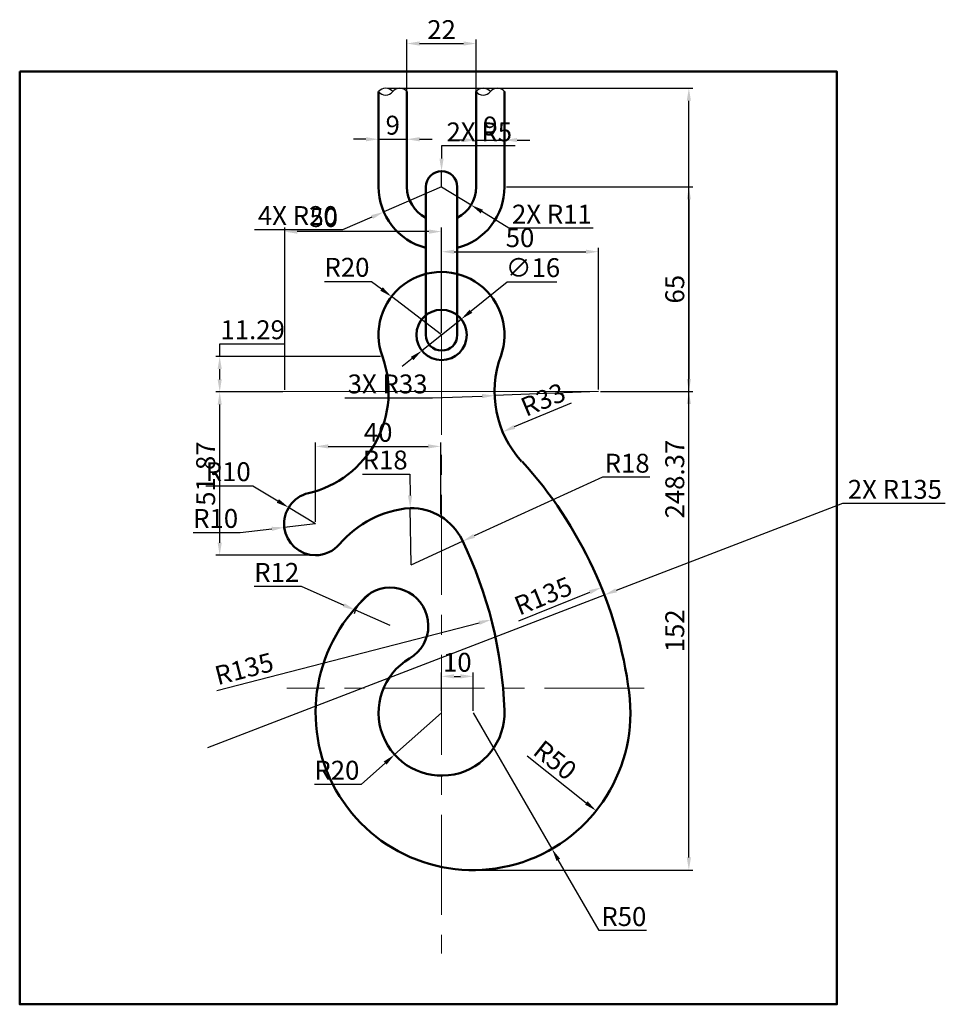
# Model space of a CAD drawing. Units: millimetres. Extents: x 103 to 397, y -55 to 258.
import ezdxf

# ---------------------------------------------------------------- set-up
doc = ezdxf.new("R2010")
doc.units = ezdxf.units.MM
doc.linetypes.add('CENTER', pattern=[50.8, 31.75, -6.35, 6.35, -6.35])
for name, color, linetype, lineweight in [('M-BRKL', 7, 'Continuous', 25), ('M-CNTR', 4, 'CENTER', 18), ('M-CONS', 8, 'Continuous', 18), ('M-DIMS', 2, 'Continuous', 25), ('M-OUTL', 7, 'Continuous', 50), ('M-TTLB', 7, 'Continuous', 50)]:
    doc.layers.add(name, color=color, linetype=linetype, lineweight=lineweight)
doc.styles.get("Standard").update_dxf_attribs({"font": 'arial.ttf'})
doc.dimstyles.new('ISO-25', dxfattribs={"dimtxt": 6, "dimasz": 4, "dimexe": 1.25, "dimexo": 0.625, "dimtad": 1, "dimtoh": 1, "dimdec": 0, "dimtxsty": 'Standard', "dimcen": 2.5, "dimadec": 0, "dimazin": 0, "dimtfac": 1, "dimtdec": 0, "dimtmove": 0, "dimatfit": 3, "dimfxl": 1, "dimarcsym": 0})

# ---------------------------------------------------------------- blocks, each defined once
blk = doc.blocks.new('*D1')
at = {"layer": 'Defpoints', "color": 0, "transparency": 16777216}
for p in [(286.8, 139.63), (256.38, 126.83)]:
    blk.add_point(p, dxfattribs=at)
at = {"layer": 'M-DIMS', "color": 0, "lineweight": -2, "transparency": 16777216}
blk.add_line((278.12, 135.98), (260.06, 128.38), dxfattribs=at)
at = {"layer": 'M-DIMS', "color": 0, "transparency": 16777216}
blk.add_solid([(259.81, 129), (260.32, 127.77), (256.38, 126.83)], dxfattribs=at)
at = {"layer": 'M-DIMS', "color": 0, "transparency": 16777216, "insert": (269.5, 136.36), "char_height": 6, "attachment_point": 5, "rotation": 22.8118}
blk.add_mtext('R33', dxfattribs=at)
blk = doc.blocks.new('*D2')
at = {"layer": 'Defpoints', "color": 0, "transparency": 16777216}
for p in [(287.73, 77.42), (162.67, 26.58)]:
    blk.add_point(p, dxfattribs=at)
at = {"layer": 'M-DIMS', "color": 0, "lineweight": -2, "transparency": 16777216}
blk.add_line((261.52, 66.77), (284.02, 75.92), dxfattribs=at)
at = {"layer": 'M-DIMS', "color": 0, "transparency": 16777216}
blk.add_solid([(283.77, 76.53), (284.27, 75.3), (287.73, 77.42)], dxfattribs=at)
at = {"layer": 'M-DIMS', "color": 0, "transparency": 16777216, "insert": (269.53, 74.01), "char_height": 6, "attachment_point": 5, "rotation": 22.1218}
blk.add_mtext('R135', dxfattribs=at)
blk = doc.blocks.new('*D3')
at = {"layer": 'Defpoints', "color": 0, "transparency": 16777216}
for p in [(246.95, 37.63), (286.06, 6.48)]:
    blk.add_point(p, dxfattribs=at)
at = {"layer": 'M-DIMS', "color": 0, "lineweight": -2, "transparency": 16777216}
blk.add_line((264.16, 23.92), (282.93, 8.97), dxfattribs=at)
at = {"layer": 'M-DIMS', "color": 0, "transparency": 16777216}
blk.add_solid([(283.35, 9.5), (282.52, 8.45), (286.06, 6.48)], dxfattribs=at)
at = {"layer": 'M-DIMS', "color": 0, "transparency": 16777216, "insert": (272.54, 21.96), "char_height": 6, "attachment_point": 5, "rotation": 321.473}
blk.add_mtext('R50', dxfattribs=at)
blk = doc.blocks.new('*D4')
at = {"layer": 'Defpoints', "color": 0, "transparency": 16777216}
for p in [(236.95, 37.63), (222.03, 24.3)]:
    blk.add_point(p, dxfattribs=at)
at = {"layer": 'M-DIMS', "color": 0, "lineweight": -2, "transparency": 16777216}
for p, q in [((236.95, 37.63), (222.03, 24.3)), ((211.49, 14.89), (219.05, 21.64)), ((196.55, 14.89), (211.49, 14.89))]:
    blk.add_line(p, q, dxfattribs=at)
at = {"layer": 'M-DIMS', "color": 0, "transparency": 16777216}
blk.add_solid([(218.6, 22.14), (219.49, 21.14), (222.03, 24.3)], dxfattribs=at)
at = {"layer": 'M-DIMS', "color": 0, "transparency": 16777216, "insert": (203.71, 18.58), "char_height": 6, "attachment_point": 5}
blk.add_mtext('R20', dxfattribs=at)
blk = doc.blocks.new('*D5')
at = {"layer": 'Defpoints', "color": 0, "transparency": 16777216}
for p in [(188.39, 102.8), (196.95, 97.63)]:
    blk.add_point(p, dxfattribs=at)
at = {"layer": 'M-DIMS', "color": 0, "lineweight": -2, "transparency": 16777216}
for p, q in [((162.04, 109.7), (176.98, 109.7)), ((176.98, 109.7), (184.97, 104.87)), ((196.95, 97.63), (188.39, 102.8))]:
    blk.add_line(p, q, dxfattribs=at)
at = {"layer": 'M-DIMS', "color": 0, "transparency": 16777216}
blk.add_solid([(185.31, 105.44), (184.62, 104.3), (188.39, 102.8)], dxfattribs=at)
at = {"layer": 'M-DIMS', "color": 0, "transparency": 16777216, "insert": (169.2, 113.39), "char_height": 6, "attachment_point": 5}
blk.add_mtext('R10', dxfattribs=at)
blk = doc.blocks.new('*D6')
at = {"layer": 'Defpoints', "color": 0, "transparency": 16777216}
for p in [(243.64, 92.1), (227.27, 84.63)]:
    blk.add_point(p, dxfattribs=at)
at = {"layer": 'M-DIMS', "color": 0, "lineweight": -2, "transparency": 16777216}
for p, q in [((288.1, 112.4), (247.28, 93.76)), ((303.07, 112.4), (288.1, 112.4)), ((227.27, 84.63), (243.64, 92.1))]:
    blk.add_line(p, q, dxfattribs=at)
blk.add_arc((227.27, 84.63), 18, 20.5586, 25.8976, dxfattribs=at)
at = {"layer": 'M-DIMS', "color": 0, "transparency": 16777216}
blk.add_solid([(247.01, 94.37), (247.56, 93.16), (243.64, 92.1)], dxfattribs=at)
at = {"layer": 'M-DIMS', "color": 0, "transparency": 16777216, "insert": (295.9, 116.09), "char_height": 6, "attachment_point": 5}
blk.add_mtext('R18', dxfattribs=at)
blk = doc.blocks.new('*D7')
at = {"layer": 'Defpoints', "color": 0, "transparency": 16777216}
for p in [(246.95, 49.17), (236.95, 37.63), (246.95, 37.63)]:
    blk.add_point(p, dxfattribs=at)
at = {"layer": 'M-DIMS', "color": 0, "lineweight": -2, "transparency": 16777216}
for p, q in [((236.95, 38.25), (236.95, 50.42)), ((246.95, 38.25), (246.95, 50.42)), ((240.95, 49.17), (242.95, 49.17))]:
    blk.add_line(p, q, dxfattribs=at)
at = {"layer": 'M-DIMS', "color": 0, "transparency": 16777216}
for points in [[(240.95, 49.84), (240.95, 48.5), (236.95, 49.17)], [(242.95, 49.84), (242.95, 48.5), (246.95, 49.17)]]:
    blk.add_solid(points, dxfattribs=at)
at = {"layer": 'M-DIMS', "color": 0, "transparency": 16777216, "insert": (241.95, 52.86), "char_height": 6, "attachment_point": 5}
blk.add_mtext('10', dxfattribs=at)
blk = doc.blocks.new('*D8')
at = {"layer": 'Defpoints', "color": 0, "transparency": 16777216}
for p in [(216.95, 219.76), (225.95, 219.76), (225.95, 219.76)]:
    blk.add_point(p, dxfattribs=at)
at = {"layer": 'M-DIMS', "color": 0, "lineweight": -2, "transparency": 16777216}
for p, q in [((212.95, 219.76), (208.95, 219.76)), ((216.95, 220.39), (216.95, 221.01)), ((216.95, 219.76), (225.95, 219.76)), ((225.95, 220.39), (225.95, 221.01)), ((229.95, 219.76), (233.95, 219.76))]:
    blk.add_line(p, q, dxfattribs=at)
at = {"layer": 'M-DIMS', "color": 0, "transparency": 16777216}
for points in [[(212.95, 220.43), (212.95, 219.09), (216.95, 219.76)], [(229.95, 220.43), (229.95, 219.09), (225.95, 219.76)]]:
    blk.add_solid(points, dxfattribs=at)
at = {"layer": 'M-DIMS', "color": 0, "transparency": 16777216, "insert": (221.45, 223.45), "char_height": 6, "attachment_point": 5}
blk.add_mtext('9', dxfattribs=at)
blk = doc.blocks.new('*D9')
at = {"layer": 'Defpoints', "color": 0, "transparency": 16777216}
for p in [(247.95, 219.76), (256.95, 219.76), (256.95, 219.5)]:
    blk.add_point(p, dxfattribs=at)
at = {"layer": 'M-DIMS', "color": 0, "lineweight": -2, "transparency": 16777216}
for p, q in [((243.95, 219.5), (239.95, 219.5)), ((247.95, 219.5), (256.95, 219.5)), ((247.95, 219.14), (247.95, 218.25)), ((256.95, 219.14), (256.95, 218.25)), ((260.95, 219.5), (264.95, 219.5))]:
    blk.add_line(p, q, dxfattribs=at)
at = {"layer": 'M-DIMS', "color": 0, "transparency": 16777216}
for points in [[(243.95, 220.17), (243.95, 218.84), (247.95, 219.5)], [(260.95, 220.17), (260.95, 218.84), (256.95, 219.5)]]:
    blk.add_solid(points, dxfattribs=at)
at = {"layer": 'M-DIMS', "color": 0, "transparency": 16777216, "insert": (252.45, 223.19), "char_height": 6, "attachment_point": 5}
blk.add_mtext('9', dxfattribs=at)
blk = doc.blocks.new('*D10')
at = {"layer": 'Defpoints', "color": 0, "transparency": 16777216}
for p in [(243.19, 162.63), (230.7, 152.62)]:
    blk.add_point(p, dxfattribs=at)
at = {"layer": 'M-DIMS', "color": 0, "lineweight": -2, "transparency": 16777216}
for p, q in [((257.81, 174.36), (246.31, 165.13)), ((273.55, 174.36), (257.81, 174.36)), ((230.7, 152.62), (243.19, 162.63)), ((227.58, 150.12), (224.46, 147.62))]:
    blk.add_line(p, q, dxfattribs=at)
at = {"layer": 'M-DIMS', "color": 0, "transparency": 16777216}
for points in [[(245.89, 165.65), (246.72, 164.61), (243.19, 162.63)], [(227.17, 150.64), (228, 149.6), (230.7, 152.62)]]:
    blk.add_solid(points, dxfattribs=at)
at = {"layer": 'M-DIMS', "color": 0, "transparency": 16777216, "insert": (265.99, 178.21), "char_height": 6, "attachment_point": 5}
blk.add_mtext('∅16', dxfattribs=at)
blk = doc.blocks.new('*D11')
at = {"layer": 'Defpoints', "color": 0, "transparency": 16777216}
for p in [(221.05, 169.77), (236.95, 157.63)]:
    blk.add_point(p, dxfattribs=at)
at = {"layer": 'M-DIMS', "color": 0, "lineweight": -2, "transparency": 16777216}
for p, q in [((199.75, 174.62), (214.7, 174.62)), ((214.7, 174.62), (217.87, 172.2)), ((236.95, 157.63), (221.05, 169.77))]:
    blk.add_line(p, q, dxfattribs=at)
at = {"layer": 'M-DIMS', "color": 0, "transparency": 16777216}
blk.add_solid([(218.28, 172.73), (217.47, 171.67), (221.05, 169.77)], dxfattribs=at)
at = {"layer": 'M-DIMS', "color": 0, "transparency": 16777216, "insert": (206.91, 178.31), "char_height": 6, "attachment_point": 5}
blk.add_mtext('R20', dxfattribs=at)
blk = doc.blocks.new('*D12')
at = {"layer": 'Defpoints', "color": 0, "transparency": 16777216}
for p in [(236.68, 122.21), (196.95, 97.63), (236.68, 99.97)]:
    blk.add_point(p, dxfattribs=at)
at = {"layer": 'M-DIMS', "color": 0, "lineweight": -2, "transparency": 16777216}
for p, q in [((196.95, 98.25), (196.95, 123.46)), ((200.95, 122.21), (232.68, 122.21)), ((236.68, 100.59), (236.68, 123.46))]:
    blk.add_line(p, q, dxfattribs=at)
at = {"layer": 'M-DIMS', "color": 0, "transparency": 16777216}
for points in [[(200.95, 122.88), (200.95, 121.54), (196.95, 122.21)], [(232.68, 122.88), (232.68, 121.54), (236.68, 122.21)]]:
    blk.add_solid(points, dxfattribs=at)
at = {"layer": 'M-DIMS', "color": 0, "transparency": 16777216, "insert": (216.81, 125.9), "char_height": 6, "attachment_point": 5}
blk.add_mtext('40', dxfattribs=at)
blk = doc.blocks.new('*D13')
at = {"layer": 'Defpoints', "color": 0, "transparency": 16777216}
for p in [(286.8, 184.04), (236.95, 157.63), (286.8, 139.63)]:
    blk.add_point(p, dxfattribs=at)
at = {"layer": 'M-DIMS', "color": 0, "lineweight": -2, "transparency": 16777216}
for p, q in [((236.95, 158.25), (236.95, 185.29)), ((286.8, 140.25), (286.8, 185.29)), ((240.95, 184.04), (282.8, 184.04))]:
    blk.add_line(p, q, dxfattribs=at)
at = {"layer": 'M-DIMS', "color": 0, "transparency": 16777216}
for points in [[(240.95, 184.7), (240.95, 183.37), (236.95, 184.04)], [(282.8, 184.7), (282.8, 183.37), (286.8, 184.04)]]:
    blk.add_solid(points, dxfattribs=at)
at = {"layer": 'M-DIMS', "color": 0, "transparency": 16777216, "insert": (261.87, 187.72), "char_height": 6, "attachment_point": 5}
blk.add_mtext('50', dxfattribs=at)
blk = doc.blocks.new('*D14')
at = {"layer": 'Defpoints', "color": 0, "transparency": 16777216}
for p in [(187.14, 190.43), (236.95, 157.63), (187.14, 139.49)]:
    blk.add_point(p, dxfattribs=at)
at = {"layer": 'M-DIMS', "color": 0, "lineweight": -2, "transparency": 16777216}
for p, q in [((187.14, 140.12), (187.14, 191.68)), ((236.95, 158.25), (236.95, 191.68)), ((232.95, 190.43), (191.14, 190.43))]:
    blk.add_line(p, q, dxfattribs=at)
at = {"layer": 'M-DIMS', "color": 0, "transparency": 16777216}
for points in [[(191.14, 191.09), (191.14, 189.76), (187.14, 190.43)], [(232.95, 191.09), (232.95, 189.76), (236.95, 190.43)]]:
    blk.add_solid(points, dxfattribs=at)
at = {"layer": 'M-DIMS', "color": 0, "transparency": 16777216, "insert": (199.54, 194.12), "char_height": 6, "attachment_point": 5}
blk.add_mtext('50', dxfattribs=at)
blk = doc.blocks.new('*D15')
at = {"layer": 'Defpoints', "color": 0, "transparency": 16777216}
for p in [(209.6, 70.15), (220.65, 65.27)]:
    blk.add_point(p, dxfattribs=at)
at = {"layer": 'M-DIMS', "color": 0, "lineweight": -2, "transparency": 16777216}
for p, q in [((177.45, 77.77), (192.35, 77.77)), ((192.35, 77.77), (205.94, 71.77)), ((220.65, 65.27), (209.6, 70.15))]:
    blk.add_line(p, q, dxfattribs=at)
blk.add_arc((220.65, 65.27), 12.09, 123.4798, 162.0881, dxfattribs=at)
at = {"layer": 'M-DIMS', "color": 0, "transparency": 16777216}
blk.add_solid([(206.21, 72.38), (205.67, 71.16), (209.6, 70.15)], dxfattribs=at)
at = {"layer": 'M-DIMS', "color": 0, "transparency": 16777216, "insert": (184.59, 81.41), "char_height": 6, "attachment_point": 5}
blk.add_mtext('R12', dxfattribs=at)
blk = doc.blocks.new('*D16')
at = {"layer": 'Defpoints', "color": 0, "transparency": 16777216}
for p in [(252.76, 67.17), (122.02, 33.53)]:
    blk.add_point(p, dxfattribs=at)
at = {"layer": 'M-DIMS', "color": 0, "lineweight": -2, "transparency": 16777216}
blk.add_line((165.54, 44.72), (248.89, 66.17), dxfattribs=at)
at = {"layer": 'M-DIMS', "color": 0, "transparency": 16777216}
blk.add_solid([(248.72, 66.82), (249.05, 65.53), (252.76, 67.17)], dxfattribs=at)
at = {"layer": 'M-DIMS', "color": 0, "transparency": 16777216, "insert": (174.44, 50.83), "char_height": 6, "attachment_point": 5, "rotation": 14.4308}
blk.add_mtext('R135', dxfattribs=at)
blk = doc.blocks.new('FORK-ARM-BREAK-9')
for centre, start, end in [((2.25, -0.61), 37.4068, 142.5932), ((2.25, 2.83), 217.4068, 322.5932), ((6.75, -0.61), 37.4068, 142.5932)]:
    blk.add_arc(centre, 2.83, start, end)
blk = doc.blocks.new('*D18')
at = {"layer": 'Defpoints', "color": 0, "transparency": 16777216}
for p in [(219.2, 236.01), (315.49, 236.01), (245.57, -12.36)]:
    blk.add_point(p, dxfattribs=at)
at = {"layer": 'M-DIMS', "color": 0, "lineweight": -2, "transparency": 16777216}
for p, q in [((219.82, 236.01), (316.74, 236.01)), ((315.49, -8.36), (315.49, 232.01)), ((246.2, -12.36), (316.74, -12.36))]:
    blk.add_line(p, q, dxfattribs=at)
at = {"layer": 'M-DIMS', "color": 0, "transparency": 16777216}
for points in [[(314.83, 232.01), (316.16, 232.01), (315.49, 236.01)], [(314.83, -8.36), (316.16, -8.36), (315.49, -12.36)]]:
    blk.add_solid(points, dxfattribs=at)
at = {"layer": 'M-DIMS', "color": 0, "transparency": 16777216, "insert": (311.8, 111.82), "char_height": 6, "attachment_point": 5, "rotation": 90}
blk.add_mtext('248.37', dxfattribs=at)
blk = doc.blocks.new('*D19')
at = {"layer": 'Defpoints', "color": 0, "transparency": 16777216}
for p in [(166.49, 139.49), (187.14, 139.49), (196.95, 87.63)]:
    blk.add_point(p, dxfattribs=at)
at = {"layer": 'M-DIMS', "color": 0, "lineweight": -2, "transparency": 16777216}
for p, q in [((186.52, 139.49), (165.24, 139.49)), ((166.49, 91.63), (166.49, 135.49)), ((196.32, 87.63), (165.24, 87.63))]:
    blk.add_line(p, q, dxfattribs=at)
at = {"layer": 'M-DIMS', "color": 0, "transparency": 16777216}
for points in [[(165.82, 135.49), (167.15, 135.49), (166.49, 139.49)], [(165.82, 91.63), (167.15, 91.63), (166.49, 87.63)]]:
    blk.add_solid(points, dxfattribs=at)
at = {"layer": 'M-DIMS', "color": 0, "transparency": 16777216, "insert": (162.8, 113.56), "char_height": 6, "attachment_point": 5, "rotation": 90}
blk.add_mtext('51.87', dxfattribs=at)
blk = doc.blocks.new('*D20')
at = {"layer": 'Defpoints', "color": 0, "transparency": 16777216}
for p in [(166.49, 150.78), (218.15, 150.78), (187.14, 139.49)]:
    blk.add_point(p, dxfattribs=at)
at = {"layer": 'M-DIMS', "color": 0, "lineweight": -2, "transparency": 16777216}
for p, q in [((166.49, 150.78), (166.49, 154.78)), ((166.49, 154.78), (186.81, 154.78)), ((217.53, 150.78), (165.24, 150.78)), ((166.49, 143.49), (166.49, 146.78)), ((186.52, 139.49), (165.24, 139.49))]:
    blk.add_line(p, q, dxfattribs=at)
at = {"layer": 'M-DIMS', "color": 0, "transparency": 16777216}
for points in [[(165.82, 146.78), (167.15, 146.78), (166.49, 150.78)], [(165.82, 143.49), (167.15, 143.49), (166.49, 139.49)]]:
    blk.add_solid(points, dxfattribs=at)
at = {"layer": 'M-DIMS', "color": 0, "transparency": 16777216, "insert": (176.96, 158.47), "char_height": 6, "attachment_point": 5}
blk.add_mtext('11.29', dxfattribs=at)
blk = doc.blocks.new('*D21')
at = {"layer": 'Defpoints', "color": 0, "transparency": 16777216}
for p in [(286.8, 139.63), (315.49, 139.63), (245.57, -12.36)]:
    blk.add_point(p, dxfattribs=at)
at = {"layer": 'M-DIMS', "color": 0, "lineweight": -2, "transparency": 16777216}
for p, q in [((287.42, 139.63), (316.74, 139.63)), ((315.49, -8.36), (315.49, 135.63)), ((246.2, -12.36), (316.74, -12.36))]:
    blk.add_line(p, q, dxfattribs=at)
at = {"layer": 'M-DIMS', "color": 0, "transparency": 16777216}
for points in [[(314.83, 135.63), (316.16, 135.63), (315.49, 139.63)], [(314.83, -8.36), (316.16, -8.36), (315.49, -12.36)]]:
    blk.add_solid(points, dxfattribs=at)
at = {"layer": 'M-DIMS', "color": 0, "transparency": 16777216, "insert": (311.8, 63.63), "char_height": 6, "attachment_point": 5, "rotation": 90}
blk.add_mtext('152', dxfattribs=at)
blk = doc.blocks.new('*D22')
at = {"layer": 'Defpoints', "color": 0, "transparency": 16777216}
for p in [(247.95, 250.16), (225.95, 204.63), (247.95, 204.63)]:
    blk.add_point(p, dxfattribs=at)
at = {"layer": 'M-DIMS', "color": 0, "lineweight": -2, "transparency": 16777216}
for p, q in [((225.95, 205.25), (225.95, 251.41)), ((247.95, 205.25), (247.95, 251.41)), ((229.95, 250.16), (243.95, 250.16))]:
    blk.add_line(p, q, dxfattribs=at)
at = {"layer": 'M-DIMS', "color": 0, "transparency": 16777216}
for points in [[(229.95, 250.83), (229.95, 249.49), (225.95, 250.16)], [(243.95, 250.83), (243.95, 249.49), (247.95, 250.16)]]:
    blk.add_solid(points, dxfattribs=at)
at = {"layer": 'M-DIMS', "color": 0, "transparency": 16777216, "insert": (236.95, 253.8), "char_height": 6, "attachment_point": 5}
blk.add_mtext('22', dxfattribs=at)
blk = doc.blocks.new('*D23')
at = {"layer": 'Defpoints', "color": 0, "transparency": 16777216}
for p in [(256.95, 204.63), (286.8, 139.63), (315.49, 139.63)]:
    blk.add_point(p, dxfattribs=at)
at = {"layer": 'M-DIMS', "color": 0, "lineweight": -2, "transparency": 16777216}
for p, q in [((257.57, 204.63), (316.74, 204.63)), ((315.49, 200.63), (315.49, 143.63)), ((287.42, 139.63), (316.74, 139.63))]:
    blk.add_line(p, q, dxfattribs=at)
at = {"layer": 'M-DIMS', "color": 0, "transparency": 16777216}
for points in [[(314.83, 200.63), (316.16, 200.63), (315.49, 204.63)], [(314.83, 143.63), (316.16, 143.63), (315.49, 139.63)]]:
    blk.add_solid(points, dxfattribs=at)
at = {"layer": 'M-DIMS', "color": 0, "transparency": 16777216, "insert": (311.8, 172.13), "char_height": 6, "attachment_point": 5, "rotation": 90}
blk.add_mtext('65', dxfattribs=at)
blk = doc.blocks.new('*D24')
at = {"layer": 'Defpoints', "color": 0, "transparency": 16777216}
for p in [(288.67, 75.03), (162.67, 26.58)]:
    blk.add_point(p, dxfattribs=at)
at = {"layer": 'M-DIMS', "color": 0, "lineweight": -2, "transparency": 16777216}
for p, q in [((364.28, 104.1), (292.41, 76.46)), ((396.94, 104.1), (364.28, 104.1)), ((162.67, 26.58), (288.67, 75.03))]:
    blk.add_line(p, q, dxfattribs=at)
at = {"layer": 'M-DIMS', "color": 0, "transparency": 16777216}
blk.add_solid([(292.17, 77.09), (292.65, 75.84), (288.67, 75.03)], dxfattribs=at)
at = {"layer": 'M-DIMS', "color": 0, "transparency": 16777216, "insert": (380.92, 107.79), "char_height": 6, "attachment_point": 5}
blk.add_mtext('2X R135', dxfattribs=at)
blk = doc.blocks.new('*D25')
at = {"layer": 'Defpoints', "color": 0, "transparency": 16777216}
for p in [(246.95, 37.63), (272.02, -5.63)]:
    blk.add_point(p, dxfattribs=at)
at = {"layer": 'M-DIMS', "color": 0, "lineweight": -2, "transparency": 16777216}
for p, q in [((246.95, 37.63), (272.02, -5.63)), ((287.06, -31.59), (274.02, -9.09)), ((302, -31.59), (287.06, -31.59))]:
    blk.add_line(p, q, dxfattribs=at)
at = {"layer": 'M-DIMS', "color": 0, "transparency": 16777216}
blk.add_solid([(274.6, -8.76), (273.45, -9.43), (272.02, -5.63)], dxfattribs=at)
at = {"layer": 'M-DIMS', "color": 0, "transparency": 16777216, "insert": (294.85, -27.9), "char_height": 6, "attachment_point": 5}
blk.add_mtext('R50', dxfattribs=at)
blk = doc.blocks.new('*D26')
at = {"layer": 'Defpoints', "color": 0, "transparency": 16777216}
for p in [(253.82, 138.34), (286.8, 139.63)]:
    blk.add_point(p, dxfattribs=at)
at = {"layer": 'M-DIMS', "color": 0, "lineweight": -2, "transparency": 16777216}
for p, q in [((234.04, 137.58), (249.82, 138.19)), ((286.8, 139.63), (253.82, 138.34)), ((206.19, 137.58), (234.04, 137.58))]:
    blk.add_line(p, q, dxfattribs=at)
at = {"layer": 'M-DIMS', "color": 0, "transparency": 16777216}
blk.add_solid([(249.8, 138.86), (249.85, 137.52), (253.82, 138.34)], dxfattribs=at)
at = {"layer": 'M-DIMS', "color": 0, "transparency": 16777216, "insert": (219.8, 141.27), "char_height": 6, "attachment_point": 5}
blk.add_mtext('3X R33', dxfattribs=at)
blk = doc.blocks.new('*D27')
at = {"layer": 'Defpoints', "color": 0, "transparency": 16777216}
for p in [(236.95, 204.63), (218.6, 196.67)]:
    blk.add_point(p, dxfattribs=at)
at = {"layer": 'M-DIMS', "color": 0, "lineweight": -2, "transparency": 16777216}
for p, q in [((236.95, 204.63), (218.6, 196.67)), ((205.63, 191.06), (214.92, 195.08)), ((177.56, 191.06), (205.63, 191.06))]:
    blk.add_line(p, q, dxfattribs=at)
at = {"layer": 'M-DIMS', "color": 0, "transparency": 16777216}
blk.add_solid([(214.66, 195.69), (215.19, 194.47), (218.6, 196.67)], dxfattribs=at)
at = {"layer": 'M-DIMS', "color": 0, "transparency": 16777216, "insert": (191.28, 194.74), "char_height": 6, "attachment_point": 5}
blk.add_mtext('4X R20', dxfattribs=at)
blk = doc.blocks.new('*D28')
at = {"layer": 'Defpoints', "color": 0, "transparency": 16777216}
for p in [(227, 102.62), (227.27, 84.63)]:
    blk.add_point(p, dxfattribs=at)
at = {"layer": 'M-DIMS', "color": 0, "lineweight": -2, "transparency": 16777216}
for p, q in [((211.86, 113.42), (226.84, 113.42)), ((226.84, 113.42), (226.94, 106.62)), ((227.27, 84.63), (227, 102.62))]:
    blk.add_line(p, q, dxfattribs=at)
at = {"layer": 'M-DIMS', "color": 0, "transparency": 16777216}
blk.add_solid([(227.61, 106.63), (226.27, 106.61), (227, 102.62)], dxfattribs=at)
at = {"layer": 'M-DIMS', "color": 0, "transparency": 16777216, "insert": (219.04, 117.11), "char_height": 6, "attachment_point": 5}
blk.add_mtext('R18', dxfattribs=at)
blk = doc.blocks.new('*D29')
at = {"layer": 'Defpoints', "color": 0, "transparency": 16777216}
for p in [(236.95, 204.63), (246.33, 198.88)]:
    blk.add_point(p, dxfattribs=at)
at = {"layer": 'M-DIMS', "color": 0, "lineweight": -2, "transparency": 16777216}
for p, q in [((236.95, 204.63), (246.33, 198.88)), ((258.29, 191.56), (249.74, 196.79)), ((285.09, 191.56), (258.29, 191.56))]:
    blk.add_line(p, q, dxfattribs=at)
at = {"layer": 'M-DIMS', "color": 0, "transparency": 16777216}
blk.add_solid([(250.09, 197.36), (249.39, 196.22), (246.33, 198.88)], dxfattribs=at)
at = {"layer": 'M-DIMS', "color": 0, "transparency": 16777216, "insert": (272, 195.2), "char_height": 6, "attachment_point": 5}
blk.add_mtext('2X R11', dxfattribs=at)
blk = doc.blocks.new('*D30')
at = {"layer": 'Defpoints', "color": 0, "transparency": 16777216}
for p in [(196.95, 97.63), (187.01, 96.48)]:
    blk.add_point(p, dxfattribs=at)
at = {"layer": 'M-DIMS', "color": 0, "lineweight": -2, "transparency": 16777216}
for p, q in [((196.95, 97.63), (187.01, 96.48)), ((158.04, 94.86), (172.98, 94.86)), ((172.98, 94.86), (183.04, 96.02))]:
    blk.add_line(p, q, dxfattribs=at)
at = {"layer": 'M-DIMS', "color": 0, "transparency": 16777216}
blk.add_solid([(182.96, 96.68), (183.11, 95.36), (187.01, 96.48)], dxfattribs=at)
at = {"layer": 'M-DIMS', "color": 0, "transparency": 16777216, "insert": (165.2, 98.55), "char_height": 6, "attachment_point": 5}
blk.add_mtext('R10', dxfattribs=at)
blk = doc.blocks.new('*D31')
at = {"layer": 'Defpoints', "color": 0, "transparency": 16777216}
for p in [(236.95, 209.63), (236.95, 204.63)]:
    blk.add_point(p, dxfattribs=at)
at = {"layer": 'M-DIMS', "color": 0, "lineweight": -2, "transparency": 16777216}
for p, q in [((260.29, 217.63), (236.95, 217.63)), ((236.95, 217.63), (236.95, 213.63)), ((236.95, 204.63), (236.95, 209.63))]:
    blk.add_line(p, q, dxfattribs=at)
at = {"layer": 'M-DIMS', "color": 0, "transparency": 16777216}
blk.add_solid([(236.28, 213.63), (237.61, 213.63), (236.95, 209.63)], dxfattribs=at)
at = {"layer": 'M-DIMS', "color": 0, "transparency": 16777216, "insert": (248.93, 221.31), "char_height": 6, "attachment_point": 5}
blk.add_mtext('2X R5', dxfattribs=at)

msp = doc.modelspace()

# ---------------------------------------------------------------- linework, layer by layer
at = {"layer": 'M-CNTR'}
for p, q in [((236.946, 157.627), (236.946, -38.856)), ((301.343, 45.421), (187.781, 45.421))]:
    msp.add_line(p, q, dxfattribs=at)
at = {"layer": 'M-CONS'}
msp.add_line((286.795, 139.627), (180.637, 139.627), dxfattribs=at)
at = {"layer": 'M-OUTL'}
for p, q in [((216.946, 204.627), (216.946, 234.897)), ((225.946, 204.627), (225.946, 234.897)), ((247.946, 204.627), (247.946, 234.897)), ((256.946, 204.627), (256.946, 234.897)), ((231.946, 157.627), (231.946, 204.627)), ((241.946, 157.627), (241.946, 204.627))]:
    msp.add_line(p, q, dxfattribs=at)
msp.add_circle((236.946, 157.627), 8, dxfattribs=at)
for centre, radius, start, end in [((236.946, 204.627), 5, 0, 180), ((236.946, 204.627), 20, 180, 255.52249), ((236.946, 204.627), 11, 180, 242.96431), ((236.946, 204.627), 11, 297.03569, 0), ((236.946, 204.627), 20, 284.47751, 0), ((236.946, 157.627), 20, 339.94745, 200.00576), ((236.946, 157.627), 5, 180, 0), ((187.144, 139.494), 33, 283.17646, 20.00576), ((286.795, 139.627), 33, 160.02568, 222.28901), ((162.666, 26.584), 135, 7.46434, 42.28901), ((196.946, 97.627), 10, 103.17646, 270), ((229.679, 69.737), 33, 94.75043, 139.60352), ((227.269, 84.627), 18, 25.89763, 91.02989), ((122.019, 33.525), 135, 2.04388, 25.89763), ((246.946, 37.627), 50, 130.43843, 7.46434), ((220.652, 65.269), 12.087, 300.51712, 120.51712), ((236.946, 37.627), 20, 120.51712, 2.04388)]:
    msp.add_arc(centre, radius, start, end, dxfattribs=at)
msp.add_open_spline([(196.946, 87.627), (199.735, 87.627), (202.74, 88.999), (204.547, 91.123)], degree=3, dxfattribs=at)
at = {"layer": 'M-TTLB'}
msp.add_lwpolyline([(102.965, 241.226), (362.531, 241.226), (362.531, -54.99), (102.965, -54.99)], close=True, dxfattribs=at)

# ---------------------------------------------------------------- block references
at = {"layer": 'M-BRKL'}
for p in [(216.946, 233.785), (247.946, 233.785)]:
    msp.add_blockref('FORK-ARM-BREAK-9', p, dxfattribs=at)

# ---------------------------------------------------------------- dimensions: what is measured, and where the dimension line sits
at = {"layer": 'M-DIMS'}
for base, p1, p2, override, picture, middle in [((247.946, 250.159), (225.946, 204.627), (247.946, 204.627), {"dimdec": 0, "dimlfac": 1, "dimrnd": 0, "dimzin": 0, "dimdsep": 46, "dimlunit": 2}, '*D22', (236.946, 253.796)), ((225.946, 219.762), (216.946, 219.762), (225.946, 219.762), {"dimclrd": 0, "dimclre": 0, "dimclrt": 0}, '*D8', (221.446, 223.45)), ((256.946, 219.504), (247.946, 219.762), (256.946, 219.762), {"dimclrd": 0, "dimclre": 0, "dimclrt": 0}, '*D9', (252.446, 223.192)), ((286.795, 184.036), (236.946, 157.627), (286.795, 139.627), {"dimclrd": 0, "dimclre": 0, "dimclrt": 0}, '*D13', (261.871, 187.724)), ((236.684, 122.21), (196.946, 97.627), (236.684, 99.968), {"dimclrd": 0, "dimclre": 0, "dimclrt": 0}, '*D12', (216.815, 125.898))]:
    dim = msp.add_linear_dim(base=base, p1=p1, p2=p2, dimstyle='ISO-25', override=override, dxfattribs=at)
    dim.commit()
    dim.dimension.update_dxf_attribs({"geometry": picture, "text_midpoint": middle})
for base, p1, p2, override, picture, middle in [((315.493, 236.009), (245.573, -12.361), (219.196, 236.009), {"dimdec": 2, "dimlfac": 1, "dimrnd": 0, "dimzin": 0, "dimdsep": 46, "dimlunit": 2}, '*D18', (311.803, 111.824)), ((315.493, 139.627), (256.946, 204.627), (286.795, 139.627), {"dimdec": 0, "dimlfac": 1, "dimrnd": 0, "dimzin": 0, "dimdsep": 46, "dimlunit": 2}, '*D23', (311.805, 172.127)), ((166.487, 150.784), (187.144, 139.494), (218.153, 150.784), {"dimdec": 2, "dimlfac": 1, "dimrnd": 0, "dimzin": 0, "dimdsep": 46, "dimlunit": 2}, '*D20', (176.959, 158.473)), ((166.487, 139.494), (196.946, 87.627), (187.144, 139.494), {"dimdec": 2, "dimlfac": 1, "dimrnd": 0, "dimzin": 0, "dimdsep": 46, "dimlunit": 2}, '*D19', (162.798, 113.561)), ((315.493, 139.627), (245.573, -12.361), (286.795, 139.627), {"dimdec": 0, "dimlfac": 1, "dimrnd": 0, "dimzin": 0, "dimdsep": 46, "dimlunit": 2}, '*D21', (311.805, 63.633))]:
    dim = msp.add_linear_dim(base=base, p1=p1, p2=p2, angle=90, dimstyle='ISO-25', override=override, dxfattribs=at)
    dim.commit()
    dim.dimension.update_dxf_attribs({"geometry": picture, "text_midpoint": middle})
for mpoint, text, picture, middle in [((236.946, 209.627), '2X <>', '*D31', (248.929, 221.315)), ((218.595, 196.674), '4X <>', '*D27', (191.283, 194.744)), ((246.327, 198.882), '2X <>', '*D29', (272.002, 195.196))]:
    dim = msp.add_radius_dim(center=(236.946, 204.627), mpoint=mpoint, text=text, dimstyle='ISO-25', override={"dimdec": 0, "dimlfac": 1, "dimrnd": 0, "dimzin": 0, "dimdsep": 46, "dimlunit": 2}, dxfattribs=at)
    dim.commit()
    dim.dimension.update_dxf_attribs({"geometry": picture, "text_midpoint": middle})
for base, p1, p2, picture, middle in [((187.144, 190.427), (236.946, 157.627), (187.144, 139.494), '*D14', (199.544, 190.427)), ((246.946, 49.171), (236.946, 37.627), (246.946, 37.627), '*D7', (241.946, 49.171))]:
    dim = msp.add_linear_dim(base=base, p1=p1, p2=p2, dimstyle='ISO-25', override={"dimclrd": 0, "dimclre": 0, "dimclrt": 0}, dxfattribs=at)
    dim.commit()
    dim.dimension.update_dxf_attribs({"geometry": picture, "text_midpoint": middle, "dimtype": 160})
for center, mpoint, override, picture, middle in [((236.946, 157.627), (221.053, 169.768), {"dimclrd": 0, "dimclre": 0, "dimclrt": 0}, '*D11', (206.912, 178.312)), ((196.946, 97.627), (187.012, 96.479), {"dimdec": 0, "dimlfac": 1, "dimrnd": 0, "dimzin": 0, "dimdsep": 46, "dimlunit": 2}, '*D30', (165.195, 98.546)), ((236.946, 37.627), (222.03, 24.303), {"dimclrd": 0, "dimclre": 0, "dimclrt": 0}, '*D4', (203.711, 18.58))]:
    dim = msp.add_radius_dim(center=center, mpoint=mpoint, dimstyle='ISO-25', override=override, dxfattribs=at)
    dim.commit()
    dim.dimension.update_dxf_attribs({"geometry": picture, "text_midpoint": middle})
dim = msp.add_diameter_dim_2p(p1=(230.704, 152.622), p2=(243.187, 162.631), dimstyle='ISO-25', override={"dimclrd": 0, "dimclre": 0, "dimclrt": 0}, dxfattribs=at)
dim.commit()
dim.dimension.update_dxf_attribs({"geometry": '*D10', "text_midpoint": (265.994, 174.356), "dimtype": 163})
for center, mpoint, text, picture, middle in [((286.795, 139.627), (253.82, 138.345), '3X <>', '*D26', (234.035, 137.576)), ((162.666, 26.584), (288.675, 75.029), '2X <>', '*D24', (380.924, 104.095))]:
    dim = msp.add_radius_dim(center=center, mpoint=mpoint, text=text, dimstyle='ISO-25', override={"dimdec": 0, "dimlfac": 1, "dimrnd": 0, "dimzin": 0, "dimdsep": 46, "dimlunit": 2}, dxfattribs=at)
    dim.commit()
    dim.dimension.update_dxf_attribs({"geometry": picture, "text_midpoint": middle, "dimtype": 164})
for center, mpoint, override, picture, middle in [((286.795, 139.627), (256.376, 126.832), {"dimclrd": 0, "dimclre": 0, "dimclrt": 0}, '*D1', (270.935, 132.956)), ((227.269, 84.627), (226.999, 102.625), {"dimdec": 0, "dimlfac": 1, "dimrnd": 0, "dimzin": 0, "dimdsep": 46, "dimlunit": 2}, '*D28', (219.038, 113.423)), ((227.269, 84.627), (243.644, 92.102), {"dimclrd": 0, "dimclre": 0, "dimclrt": 0}, '*D6', (295.899, 112.397)), ((196.946, 97.627), (188.388, 102.8), {"dimclrd": 0, "dimclre": 0, "dimclrt": 0}, '*D5', (169.198, 109.697)), ((220.652, 65.269), (209.596, 70.154), {"dimclrd": 0, "dimclre": 0, "dimclrt": 0}, '*D15', (184.588, 77.773)), ((162.666, 26.584), (287.728, 77.422), {"dimclrd": 0, "dimclre": 0, "dimclrt": 0}, '*D2', (270.917, 70.588)), ((122.019, 33.525), (252.76, 67.169), {"dimclrd": 0, "dimclre": 0, "dimclrt": 0}, '*D16', (175.363, 47.252)), ((246.946, 37.627), (286.062, 6.482), {"dimclrd": 0, "dimclre": 0, "dimclrt": 0}, '*D3', (270.246, 19.075)), ((246.946, 37.627), (272.019, -5.632), {"dimdec": 0, "dimlfac": 1, "dimrnd": 0, "dimzin": 0, "dimdsep": 46, "dimlunit": 2}, '*D25', (294.846, -31.588))]:
    dim = msp.add_radius_dim(center=center, mpoint=mpoint, dimstyle='ISO-25', override=override, dxfattribs=at)
    dim.commit()
    dim.dimension.update_dxf_attribs({"geometry": picture, "text_midpoint": middle, "dimtype": 164})

doc.saveas('drawing.dxf')
